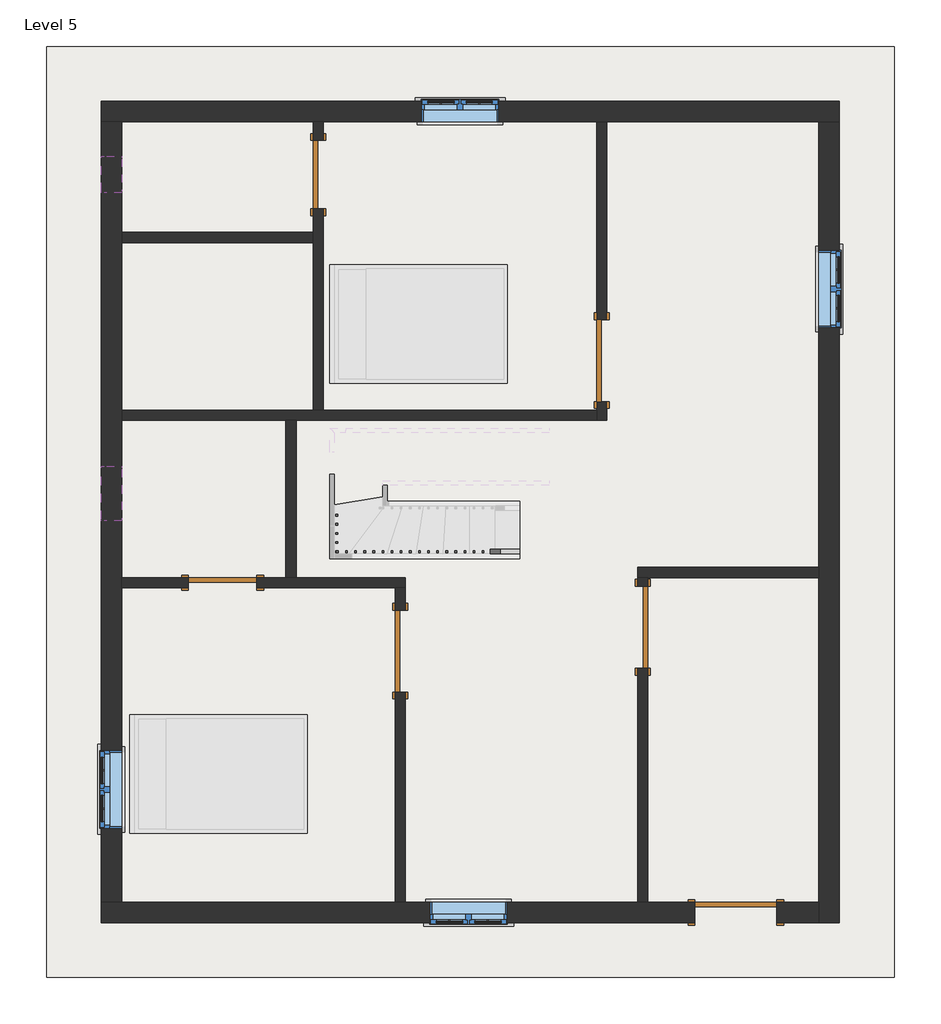
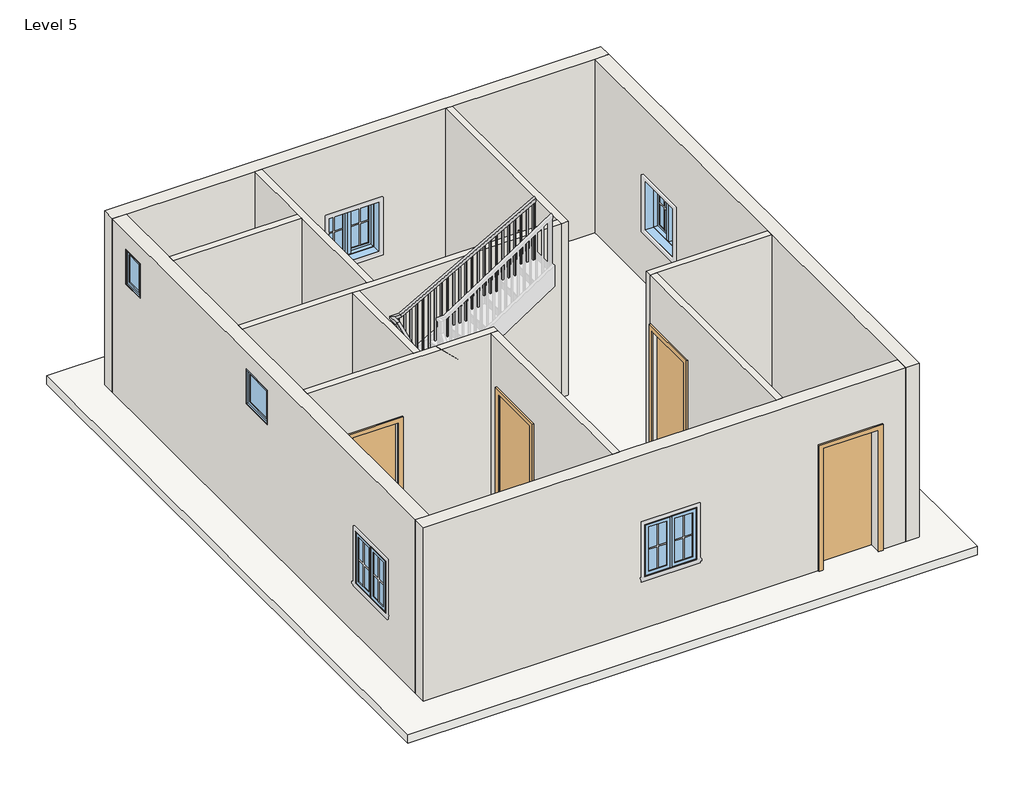
# One storey, part 1 of 2: 13 walls, 6 doors, 6 windows, 1 railing, 1 roof.
"""IFC4 building model written with IfcOpenShell, lengths in millimetres."""

from ifc_helpers import new_model, si_unit, frame, origin, place, context, project, spatial, polyline, outline, extrude, faceted_brep, transform, mapped, element, save
from components import door_d8f5dbb5, door_f2b275c1, door_305aa2a5, door_e5f9f3c4, door_0ca8825f, window_aa618e30, window_80340324, window_339605e1

model = new_model("IFC4")

# Units and contexts
model_context = context("Model", 3, world=origin())
ifc_project = project(units=[si_unit("LENGTHUNIT", "METRE", prefix="MILLI")], contexts=[model_context])

# Site, building, storey
site = spatial("IfcSite", under=ifc_project)
building = spatial("IfcBuilding", under=site)
storey = spatial("IfcBuildingStorey", under=building, Name="Level 5", Elevation=9601.2)

# Doors
placement = place(None, origin())
door_shape = door_d8f5dbb5(model_context)
element("IfcDoor", 1, ObjectType="Single-Flush : 30\" x 80\"", at=placement, inside=storey, context=model_context, shape_type="MappedRepresentation", body=[
    mapped(door_shape, transform((-2510.1648498, 3958.5558073, 9601.2), x_axis=(0.0, 1.0, 0.0), y_axis=(-1.0, 0.0, 0.0), z_axis=(0.0, 0.0, 1.0))),
])
door_2_shape = door_f2b275c1(model_context)
element("IfcDoor", 2, ObjectType="Single-Flush : 30\" x 80\"", at=placement, inside=storey, context=model_context, shape_type="MappedRepresentation", body=[
    mapped(door_2_shape, transform((-3576.9648498, -592.8066927, 9601.2), x_axis=(-1.0, 0.0, 0.0), y_axis=(0.0, -1.0, 0.0), z_axis=(0.0, 0.0, 1.0))),
])
door_3_shape = door_305aa2a5(model_context)
element("IfcDoor", 3, ObjectType="Single-Flush : 36\" x 84\"", at=placement, inside=storey, context=model_context, shape_type="MappedRepresentation", body=[
    mapped(door_3_shape, transform((652.1351502, 1883.6933073, 9601.2), x_axis=(0.0, -1.0, 0.0), y_axis=(1.0, 0.0, 0.0), z_axis=(0.0, 0.0, 1.0))),
])
element("IfcDoor", 4, ObjectType="Single-Flush : 36\" x 84\"", at=placement, inside=storey, context=model_context, shape_type="MappedRepresentation", body=[
    mapped(door_3_shape, transform((1109.3351502, -1088.1066927, 9601.2), x_axis=(0.0, 1.0, 0.0), y_axis=(-1.0, 0.0, 0.0), z_axis=(0.0, 0.0, 1.0))),
])
door_4_shape = door_e5f9f3c4(model_context)
element("IfcDoor", 5, ObjectType="Single-Flush : 36\" x 84\"", at=placement, inside=storey, context=model_context, shape_type="MappedRepresentation", body=[
    mapped(door_4_shape, transform((-1595.7648498, -1354.8066927, 9601.2), x_axis=(0.0, 1.0, 0.0), y_axis=(-1.0, 0.0, 0.0), z_axis=(0.0, 0.0, 1.0))),
])
door_5_shape = door_0ca8825f(model_context)
element("IfcDoor", 6, ObjectType="Single-Flush : 36\" x 84\"", at=placement, inside=storey, context=model_context, shape_type="MappedRepresentation", body=[
    mapped(door_5_shape, transform((2147.5601502, -4269.4566927, 9601.2), x_axis=(1.0, 0.0, 0.0), y_axis=(0.0, 1.0, 0.0), z_axis=(0.0, 0.0, 1.0))),
])

# Railing
element("IfcRailing", 7, ObjectType="Handrail - Rectangular", at=placement, inside=storey, context=model_context, shape_type="SolidModel", body=[
    faceted_brep([(-264.8831579, -271.8029286, 10684.9333333), (-264.8831579, -271.8029286, 10627.3518622), (-264.8831579, -221.0029286, 10627.3518622), (-264.8831579, -221.0029286, 10684.9333333), (-2203.3957557, -271.8029286, 11719.466441), (-2216.1029055, -271.8029286, 11668.666441), (-2216.1029055, -221.0029286, 11668.666441), (-2203.3957557, -221.0029286, 11719.466441), (-2328.8610857, -271.8029286, 11719.466441), (-2328.8610857, -271.8029286, 11668.666441), (-2278.0610857, -221.0029286, 11668.666441), (-2278.0610857, -221.0029286, 11719.466441), (-2328.8610857, -117.3180853, 11719.466441), (-2328.8610857, -107.2249429, 11668.666441), (-2278.0610857, -107.2249429, 11668.666441), (-2278.0610857, -117.3180853, 11719.466441), (-2328.8610857, 889.2076495, 12135.8648193), (-2328.8610857, 899.300792, 12085.0648193), (-2278.0610857, 899.300792, 12085.0648193), (-2278.0610857, 889.2076495, 12135.8648193), (-2328.8610857, 1080.0895433, 12135.8648193), (-2328.8610857, 1080.0895433, 12085.0648193), (-2278.0610857, 1029.2895433, 12085.0648193), (-2278.0610857, 1029.2895433, 12135.8648193), (-2181.3423106, 1080.0895433, 12135.8648193), (-2168.0744201, 1080.0895433, 12085.0648193), (-2168.0744201, 1029.2895433, 12085.0648193), (-2181.3423106, 1029.2895433, 12135.8648193), (63.4034409, 1080.0895433, 13394.2666667), (63.4034409, 1029.2895433, 13394.2666667), (63.4034409, 1029.2895433, 13336.0287027), (63.4034409, 1080.0895433, 13336.0287027)], [[[0, 1, 2, 3]], [[1, 0, 4, 5]], [[2, 1, 5, 6]], [[3, 2, 6, 7]], [[0, 3, 7, 4]], [[5, 4, 8, 9]], [[6, 5, 9, 10]], [[7, 6, 10, 11]], [[4, 7, 11, 8]], [[9, 8, 12, 13]], [[10, 9, 13, 14]], [[11, 10, 14, 15]], [[8, 11, 15, 12]], [[13, 12, 16, 17]], [[14, 13, 17, 18]], [[15, 14, 18, 19]], [[12, 15, 19, 16]], [[17, 16, 20, 21]], [[18, 17, 21, 22]], [[19, 18, 22, 23]], [[16, 19, 23, 20]], [[21, 20, 24, 25]], [[22, 21, 25, 26]], [[23, 22, 26, 27]], [[20, 23, 27, 24]], [[28, 29, 30, 31]], [[25, 24, 28, 31]], [[26, 25, 31, 30]], [[27, 26, 30, 29]], [[24, 27, 29, 28]]]),
    extrude(outline(polyline([(13313.8348603, 23.8139143), (12310.5333333, 23.8139143), (12310.5333333, 42.8639143), (13324.5142681, 42.8639143), (13313.8348603, 23.8139143)])), frame((0.0, 1045.1645433, 0.0), z_axis=(0.0, 1.0, 0.0), x_axis=(0.0, 0.0, 1.0)), (0.0, 0.0, 1.0), 19.05),
    extrude(outline(polyline([(13256.878019, -77.7860857), (12310.5333333, -77.7860857), (12310.5333333, -58.7360857), (13267.5574267, -58.7360857), (13256.878019, -77.7860857)])), frame((0.0, 1045.1645433, 0.0), z_axis=(0.0, 1.0, 0.0), x_axis=(0.0, 0.0, 1.0)), (0.0, 0.0, 1.0), 19.05),
    extrude(outline(polyline([(13199.9211776, -179.3860857), (12310.5333333, -179.3860857), (12310.5333333, -160.3360857), (13210.6005853, -160.3360857), (13199.9211776, -179.3860857)])), frame((0.0, 1045.1645433, 0.0), z_axis=(0.0, 1.0, 0.0), x_axis=(0.0, 0.0, 1.0)), (0.0, 0.0, 1.0), 19.05),
    extrude(outline(polyline([(13142.9643362, -280.9860857), (12141.2, -280.9860857), (12141.2, -261.9360857), (13153.643744, -261.9360857), (13142.9643362, -280.9860857)])), frame((0.0, 1045.1645433, 0.0), z_axis=(0.0, 1.0, 0.0), x_axis=(0.0, 0.0, 1.0)), (0.0, 0.0, 1.0), 19.05),
    extrude(outline(polyline([(13086.0074948, -382.5860857), (12141.2, -382.5860857), (12141.2, -363.5360857), (13096.6869026, -363.5360857), (13086.0074948, -382.5860857)])), frame((0.0, 1045.1645433, 0.0), z_axis=(0.0, 1.0, 0.0), x_axis=(0.0, 0.0, 1.0)), (0.0, 0.0, 1.0), 19.05),
    extrude(outline(polyline([(13029.0506535, -484.1860857), (12141.2, -484.1860857), (12141.2, -465.1360857), (13039.7300612, -465.1360857), (13029.0506535, -484.1860857)])), frame((0.0, 1045.1645433, 0.0), z_axis=(0.0, 1.0, 0.0), x_axis=(0.0, 0.0, 1.0)), (0.0, 0.0, 1.0), 19.05),
    extrude(outline(polyline([(12972.0938121, -585.7860857), (11971.8666667, -585.7860857), (11971.8666667, -566.7360857), (12982.7732198, -566.7360857), (12972.0938121, -585.7860857)])), frame((0.0, 1045.1645433, 0.0), z_axis=(0.0, 1.0, 0.0), x_axis=(0.0, 0.0, 1.0)), (0.0, 0.0, 1.0), 19.05),
    extrude(outline(polyline([(12915.1369707, -687.3860857), (11971.8666667, -687.3860857), (11971.8666667, -668.3360857), (12925.8163785, -668.3360857), (12915.1369707, -687.3860857)])), frame((0.0, 1045.1645433, 0.0), z_axis=(0.0, 1.0, 0.0), x_axis=(0.0, 0.0, 1.0)), (0.0, 0.0, 1.0), 19.05),
    extrude(outline(polyline([(12858.1801293, -788.9860857), (11971.8666667, -788.9860857), (11971.8666667, -769.9360857), (12868.8595371, -769.9360857), (12858.1801293, -788.9860857)])), frame((0.0, 1045.1645433, 0.0), z_axis=(0.0, 1.0, 0.0), x_axis=(0.0, 0.0, 1.0)), (0.0, 0.0, 1.0), 19.05),
    extrude(outline(polyline([(12801.223288, -890.5860857), (11802.5333333, -890.5860857), (11802.5333333, -871.5360857), (12811.9026957, -871.5360857), (12801.223288, -890.5860857)])), frame((0.0, 1045.1645433, 0.0), z_axis=(0.0, 1.0, 0.0), x_axis=(0.0, 0.0, 1.0)), (0.0, 0.0, 1.0), 19.05),
    extrude(outline(polyline([(12744.2664466, -992.1860857), (11802.5333333, -992.1860857), (11802.5333333, -973.1360857), (12754.9458543, -973.1360857), (12744.2664466, -992.1860857)])), frame((0.0, 1045.1645433, 0.0), z_axis=(0.0, 1.0, 0.0), x_axis=(0.0, 0.0, 1.0)), (0.0, 0.0, 1.0), 19.05),
    extrude(outline(polyline([(12687.3096052, -1093.7860857), (11633.2, -1093.7860857), (11633.2, -1074.7360857), (12697.989013, -1074.7360857), (12687.3096052, -1093.7860857)])), frame((0.0, 1045.1645433, 0.0), z_axis=(0.0, 1.0, 0.0), x_axis=(0.0, 0.0, 1.0)), (0.0, 0.0, 1.0), 19.05),
    extrude(outline(polyline([(12630.3527638, -1195.3860857), (11633.2, -1195.3860857), (11633.2, -1176.3360857), (12641.0321716, -1176.3360857), (12630.3527638, -1195.3860857)])), frame((0.0, 1045.1645433, 0.0), z_axis=(0.0, 1.0, 0.0), x_axis=(0.0, 0.0, 1.0)), (0.0, 0.0, 1.0), 19.05),
    extrude(outline(polyline([(12573.3959225, -1296.9860857), (11633.2, -1296.9860857), (11633.2, -1277.9360857), (12584.0753302, -1277.9360857), (12573.3959225, -1296.9860857)])), frame((0.0, 1045.1645433, 0.0), z_axis=(0.0, 1.0, 0.0), x_axis=(0.0, 0.0, 1.0)), (0.0, 0.0, 1.0), 19.05),
    extrude(outline(polyline([(12516.4390811, -1398.5860857), (11463.8666667, -1398.5860857), (11463.8666667, -1379.5360857), (12527.1184889, -1379.5360857), (12516.4390811, -1398.5860857)])), frame((0.0, 1045.1645433, 0.0), z_axis=(0.0, 1.0, 0.0), x_axis=(0.0, 0.0, 1.0)), (0.0, 0.0, 1.0), 19.05),
    extrude(outline(polyline([(12459.4822397, -1500.1860857), (11463.8666667, -1500.1860857), (11463.8666667, -1481.1360857), (12470.1616475, -1481.1360857), (12459.4822397, -1500.1860857)])), frame((0.0, 1045.1645433, 0.0), z_axis=(0.0, 1.0, 0.0), x_axis=(0.0, 0.0, 1.0)), (0.0, 0.0, 1.0), 19.05),
    extrude(outline(polyline([(12402.5253983, -1601.7860857), (11463.8666667, -1601.7860857), (11463.8666667, -1582.7360857), (12413.2048061, -1582.7360857), (12402.5253983, -1601.7860857)])), frame((0.0, 1045.1645433, 0.0), z_axis=(0.0, 1.0, 0.0), x_axis=(0.0, 0.0, 1.0)), (0.0, 0.0, 1.0), 19.05),
    extrude(outline(polyline([(12345.568557, -1703.3860857), (11294.5333333, -1703.3860857), (11294.5333333, -1684.3360857), (12356.2479647, -1684.3360857), (12345.568557, -1703.3860857)])), frame((0.0, 1045.1645433, 0.0), z_axis=(0.0, 1.0, 0.0), x_axis=(0.0, 0.0, 1.0)), (0.0, 0.0, 1.0), 19.05),
    extrude(outline(polyline([(12288.6117156, -1804.9860857), (11294.5333333, -1804.9860857), (11294.5333333, -1785.9360857), (12299.2911234, -1785.9360857), (12288.6117156, -1804.9860857)])), frame((0.0, 1045.1645433, 0.0), z_axis=(0.0, 1.0, 0.0), x_axis=(0.0, 0.0, 1.0)), (0.0, 0.0, 1.0), 19.05),
    extrude(outline(polyline([(12231.6548742, -1906.5860857), (11294.5333333, -1906.5860857), (11294.5333333, -1887.5360857), (12242.334282, -1887.5360857), (12231.6548742, -1906.5860857)])), frame((0.0, 1045.1645433, 0.0), z_axis=(0.0, 1.0, 0.0), x_axis=(0.0, 0.0, 1.0)), (0.0, 0.0, 1.0), 19.05),
    extrude(outline(polyline([(12174.6980329, -2008.1860857), (11294.5333333, -2008.1860857), (11294.5333333, -1989.1360857), (12185.3774406, -1989.1360857), (12174.6980329, -2008.1860857)])), frame((0.0, 1045.1645433, 0.0), z_axis=(0.0, 1.0, 0.0), x_axis=(0.0, 0.0, 1.0)), (0.0, 0.0, 1.0), 19.05),
    extrude(outline(polyline([(12117.7411915, -2109.7860857), (11125.2, -2109.7860857), (11125.2, -2090.7360857), (12128.4205992, -2090.7360857), (12117.7411915, -2109.7860857)])), frame((0.0, 1045.1645433, 0.0), z_axis=(0.0, 1.0, 0.0), x_axis=(0.0, 0.0, 1.0)), (0.0, 0.0, 1.0), 19.05),
    extrude(outline(polyline([(-2211.3860857, 1064.2145433), (-2192.3360857, 1064.2145433), (-2192.3360857, 1045.1645433), (-2211.3860857, 1045.1645433), (-2211.3860857, 1064.2145433)])), frame((0.0, 0.0, 11125.2), z_axis=(0.0, 0.0, 1.0), x_axis=(1.0, 0.0, 0.0)), (0.0, 0.0, 1.0), 959.8648193),
    extrude(outline(polyline([(-2312.9860857, 963.2720714), (-2312.9860857, 982.3220714), (-2293.9360857, 982.3220714), (-2293.9360857, 963.2720714), (-2312.9860857, 963.2720714)])), frame((0.0, 0.0, 11125.2), z_axis=(0.0, 0.0, 1.0), x_axis=(1.0, 0.0, 0.0)), (0.0, 0.0, 1.0), 959.8648193),
    extrude(outline(polyline([(880.7220714, 12077.3788269), (880.7220714, 11125.2), (861.6720714, 11125.2), (861.6720714, 12069.4978669), (880.7220714, 12077.3788269)])), frame((-2312.9860857, 0.0, 0.0), z_axis=(1.0, 0.0, 0.0), x_axis=(0.0, 1.0, 0.0)), (0.0, 0.0, 1.0), 19.05),
    extrude(outline(polyline([(779.1220714, 12035.34704), (779.1220714, 11125.2), (760.0720714, 11125.2), (760.0720714, 12027.4660799), (779.1220714, 12035.34704)])), frame((-2312.9860857, 0.0, 0.0), z_axis=(1.0, 0.0, 0.0), x_axis=(0.0, 1.0, 0.0)), (0.0, 0.0, 1.0), 19.05),
    extrude(outline(polyline([(677.5220714, 11993.315253), (677.5220714, 11125.2), (658.4720714, 11125.2), (658.4720714, 11985.434293), (677.5220714, 11993.315253)])), frame((-2312.9860857, 0.0, 0.0), z_axis=(1.0, 0.0, 0.0), x_axis=(0.0, 1.0, 0.0)), (0.0, 0.0, 1.0), 19.05),
    extrude(outline(polyline([(575.9220714, 11951.2834661), (575.9220714, 10955.8666667), (556.8720714, 10955.8666667), (556.8720714, 11943.402506), (575.9220714, 11951.2834661)])), frame((-2312.9860857, 0.0, 0.0), z_axis=(1.0, 0.0, 0.0), x_axis=(0.0, 1.0, 0.0)), (0.0, 0.0, 1.0), 19.05),
    extrude(outline(polyline([(474.3220714, 11909.2516792), (474.3220714, 10955.8666667), (455.2720714, 10955.8666667), (455.2720714, 11901.3707191), (474.3220714, 11909.2516792)])), frame((-2312.9860857, 0.0, 0.0), z_axis=(1.0, 0.0, 0.0), x_axis=(0.0, 1.0, 0.0)), (0.0, 0.0, 1.0), 19.05),
    extrude(outline(polyline([(372.7220714, 11867.2198922), (372.7220714, 10955.8666667), (353.6720714, 10955.8666667), (353.6720714, 11859.3389322), (372.7220714, 11867.2198922)])), frame((-2312.9860857, 0.0, 0.0), z_axis=(1.0, 0.0, 0.0), x_axis=(0.0, 1.0, 0.0)), (0.0, 0.0, 1.0), 19.05),
    extrude(outline(polyline([(271.1220714, 11825.1881053), (271.1220714, 10955.8666667), (252.0720714, 10955.8666667), (252.0720714, 11817.3071452), (271.1220714, 11825.1881053)])), frame((-2312.9860857, 0.0, 0.0), z_axis=(1.0, 0.0, 0.0), x_axis=(0.0, 1.0, 0.0)), (0.0, 0.0, 1.0), 19.05),
    extrude(outline(polyline([(169.5220714, 11783.1563183), (169.5220714, 10786.5333333), (150.4720714, 10786.5333333), (150.4720714, 11775.2753583), (169.5220714, 11783.1563183)])), frame((-2312.9860857, 0.0, 0.0), z_axis=(1.0, 0.0, 0.0), x_axis=(0.0, 1.0, 0.0)), (0.0, 0.0, 1.0), 19.05),
    extrude(outline(polyline([(67.9220714, 11741.1245314), (67.9220714, 10786.5333333), (48.8720714, 10786.5333333), (48.8720714, 11733.2435714), (67.9220714, 11741.1245314)])), frame((-2312.9860857, 0.0, 0.0), z_axis=(1.0, 0.0, 0.0), x_axis=(0.0, 1.0, 0.0)), (0.0, 0.0, 1.0), 19.05),
    extrude(outline(polyline([(-33.6779286, 11699.0927445), (-33.6779286, 10786.5333333), (-52.7279286, 10786.5333333), (-52.7279286, 11691.2117844), (-33.6779286, 11699.0927445)])), frame((-2312.9860857, 0.0, 0.0), z_axis=(1.0, 0.0, 0.0), x_axis=(0.0, 1.0, 0.0)), (0.0, 0.0, 1.0), 19.05),
    extrude(outline(polyline([(-2312.9860857, -154.3279286), (-2312.9860857, -135.2779286), (-2293.9360857, -135.2779286), (-2293.9360857, -154.3279286), (-2312.9860857, -154.3279286)])), frame((0.0, 0.0, 10786.5333333), z_axis=(0.0, 0.0, 1.0), x_axis=(1.0, 0.0, 0.0)), (0.0, 0.0, 1.0), 882.1331077),
    extrude(outline(polyline([(-2287.3581579, -255.9279286), (-2306.4081579, -255.9279286), (-2306.4081579, -236.8779286), (-2287.3581579, -236.8779286), (-2287.3581579, -255.9279286)])), frame((0.0, 0.0, 10786.5333333), z_axis=(0.0, 0.0, 1.0), x_axis=(1.0, 0.0, 0.0)), (0.0, 0.0, 1.0), 882.1331077),
    extrude(outline(polyline([(11662.6387317, -2204.8081579), (10786.5333333, -2204.8081579), (10786.5333333, -2185.7581579), (11652.4722486, -2185.7581579), (11662.6387317, -2204.8081579)])), frame((0.0, -255.9279286, 0.0), z_axis=(0.0, 1.0, 0.0), x_axis=(0.0, 0.0, 1.0)), (0.0, 0.0, 1.0), 19.05),
    extrude(outline(polyline([(11608.4174882, -2103.2081579), (10617.2, -2103.2081579), (10617.2, -2084.1581579), (11598.251005, -2084.1581579), (11608.4174882, -2103.2081579)])), frame((0.0, -255.9279286, 0.0), z_axis=(0.0, 1.0, 0.0), x_axis=(0.0, 0.0, 1.0)), (0.0, 0.0, 1.0), 19.05),
    extrude(outline(polyline([(11554.1962446, -2001.6081579), (10617.2, -2001.6081579), (10617.2, -1982.5581579), (11544.0297614, -1982.5581579), (11554.1962446, -2001.6081579)])), frame((0.0, -255.9279286, 0.0), z_axis=(0.0, 1.0, 0.0), x_axis=(0.0, 0.0, 1.0)), (0.0, 0.0, 1.0), 19.05),
    extrude(outline(polyline([(11499.975001, -1900.0081579), (10617.2, -1900.0081579), (10617.2, -1880.9581579), (11489.8085178, -1880.9581579), (11499.975001, -1900.0081579)])), frame((0.0, -255.9279286, 0.0), z_axis=(0.0, 1.0, 0.0), x_axis=(0.0, 0.0, 1.0)), (0.0, 0.0, 1.0), 19.05),
    extrude(outline(polyline([(11445.7537574, -1798.4081579), (10617.2, -1798.4081579), (10617.2, -1779.3581579), (11435.5872743, -1779.3581579), (11445.7537574, -1798.4081579)])), frame((0.0, -255.9279286, 0.0), z_axis=(0.0, 1.0, 0.0), x_axis=(0.0, 0.0, 1.0)), (0.0, 0.0, 1.0), 19.05),
    extrude(outline(polyline([(11391.5325139, -1696.8081579), (10447.8666667, -1696.8081579), (10447.8666667, -1677.7581579), (11381.3660307, -1677.7581579), (11391.5325139, -1696.8081579)])), frame((0.0, -255.9279286, 0.0), z_axis=(0.0, 1.0, 0.0), x_axis=(0.0, 0.0, 1.0)), (0.0, 0.0, 1.0), 19.05),
    extrude(outline(polyline([(11337.3112703, -1595.2081579), (10447.8666667, -1595.2081579), (10447.8666667, -1576.1581579), (11327.1447871, -1576.1581579), (11337.3112703, -1595.2081579)])), frame((0.0, -255.9279286, 0.0), z_axis=(0.0, 1.0, 0.0), x_axis=(0.0, 0.0, 1.0)), (0.0, 0.0, 1.0), 19.05),
    extrude(outline(polyline([(11283.0900267, -1493.6081579), (10447.8666667, -1493.6081579), (10447.8666667, -1474.5581579), (11272.9235435, -1474.5581579), (11283.0900267, -1493.6081579)])), frame((0.0, -255.9279286, 0.0), z_axis=(0.0, 1.0, 0.0), x_axis=(0.0, 0.0, 1.0)), (0.0, 0.0, 1.0), 19.05),
    extrude(outline(polyline([(11228.8687831, -1392.0081579), (10278.5333333, -1392.0081579), (10278.5333333, -1372.9581579), (11218.7023, -1372.9581579), (11228.8687831, -1392.0081579)])), frame((0.0, -255.9279286, 0.0), z_axis=(0.0, 1.0, 0.0), x_axis=(0.0, 0.0, 1.0)), (0.0, 0.0, 1.0), 19.05),
    extrude(outline(polyline([(11174.6475396, -1290.4081579), (10278.5333333, -1290.4081579), (10278.5333333, -1271.3581579), (11164.4810564, -1271.3581579), (11174.6475396, -1290.4081579)])), frame((0.0, -255.9279286, 0.0), z_axis=(0.0, 1.0, 0.0), x_axis=(0.0, 0.0, 1.0)), (0.0, 0.0, 1.0), 19.05),
    extrude(outline(polyline([(11120.426296, -1188.8081579), (10278.5333333, -1188.8081579), (10278.5333333, -1169.7581579), (11110.2598128, -1169.7581579), (11120.426296, -1188.8081579)])), frame((0.0, -255.9279286, 0.0), z_axis=(0.0, 1.0, 0.0), x_axis=(0.0, 0.0, 1.0)), (0.0, 0.0, 1.0), 19.05),
    extrude(outline(polyline([(11066.2050524, -1087.2081579), (10109.2, -1087.2081579), (10109.2, -1068.1581579), (11056.0385692, -1068.1581579), (11066.2050524, -1087.2081579)])), frame((0.0, -255.9279286, 0.0), z_axis=(0.0, 1.0, 0.0), x_axis=(0.0, 0.0, 1.0)), (0.0, 0.0, 1.0), 19.05),
    extrude(outline(polyline([(11011.9838088, -985.6081579), (10109.2, -985.6081579), (10109.2, -966.5581579), (11001.8173257, -966.5581579), (11011.9838088, -985.6081579)])), frame((0.0, -255.9279286, 0.0), z_axis=(0.0, 1.0, 0.0), x_axis=(0.0, 0.0, 1.0)), (0.0, 0.0, 1.0), 19.05),
    extrude(outline(polyline([(10957.7625653, -884.0081579), (10109.2, -884.0081579), (10109.2, -864.9581579), (10947.5960821, -864.9581579), (10957.7625653, -884.0081579)])), frame((0.0, -255.9279286, 0.0), z_axis=(0.0, 1.0, 0.0), x_axis=(0.0, 0.0, 1.0)), (0.0, 0.0, 1.0), 19.05),
    extrude(outline(polyline([(10903.5413217, -782.4081579), (9939.8666667, -782.4081579), (9939.8666667, -763.3581579), (10893.3748385, -763.3581579), (10903.5413217, -782.4081579)])), frame((0.0, -255.9279286, 0.0), z_axis=(0.0, 1.0, 0.0), x_axis=(0.0, 0.0, 1.0)), (0.0, 0.0, 1.0), 19.05),
    extrude(outline(polyline([(10849.3200781, -680.8081579), (9939.8666667, -680.8081579), (9939.8666667, -661.7581579), (10839.1535949, -661.7581579), (10849.3200781, -680.8081579)])), frame((0.0, -255.9279286, 0.0), z_axis=(0.0, 1.0, 0.0), x_axis=(0.0, 0.0, 1.0)), (0.0, 0.0, 1.0), 19.05),
    extrude(outline(polyline([(10795.0988345, -579.2081579), (9939.8666667, -579.2081579), (9939.8666667, -560.1581579), (10784.9323514, -560.1581579), (10795.0988345, -579.2081579)])), frame((0.0, -255.9279286, 0.0), z_axis=(0.0, 1.0, 0.0), x_axis=(0.0, 0.0, 1.0)), (0.0, 0.0, 1.0), 19.05),
    extrude(outline(polyline([(10740.877591, -477.6081579), (9770.5333333, -477.6081579), (9770.5333333, -458.5581579), (10730.7111078, -458.5581579), (10740.877591, -477.6081579)])), frame((0.0, -255.9279286, 0.0), z_axis=(0.0, 1.0, 0.0), x_axis=(0.0, 0.0, 1.0)), (0.0, 0.0, 1.0), 19.05),
    extrude(outline(polyline([(10686.6563474, -376.0081579), (9770.5333333, -376.0081579), (9770.5333333, -356.9581579), (10676.4898642, -356.9581579), (10686.6563474, -376.0081579)])), frame((0.0, -255.9279286, 0.0), z_axis=(0.0, 1.0, 0.0), x_axis=(0.0, 0.0, 1.0)), (0.0, 0.0, 1.0), 19.05),
    extrude(outline(polyline([(-2312.9860857, 1045.1645433), (-2312.9860857, 1064.2145433), (-2293.9360857, 1064.2145433), (-2293.9360857, 1045.1645433), (-2312.9860857, 1045.1645433)])), frame((0.0, 0.0, 11125.2), z_axis=(0.0, 0.0, 1.0), x_axis=(1.0, 0.0, 0.0)), (0.0, 0.0, 1.0), 959.8648193),
    extrude(outline(polyline([(-2293.9360857, -255.9279286), (-2312.9860857, -255.9279286), (-2312.9860857, -236.8779286), (-2293.9360857, -236.8779286), (-2293.9360857, -255.9279286)])), frame((0.0, 0.0, 10786.5333333), z_axis=(0.0, 0.0, 1.0), x_axis=(1.0, 0.0, 0.0)), (0.0, 0.0, 1.0), 882.1331077),
    extrude(outline(polyline([(13325.349295, 44.3534409), (12310.5333333, 44.3534409), (12310.5333333, 63.4034409), (13336.0287027, 63.4034409), (13325.349295, 44.3534409)])), frame((0.0, 1045.1645433, 0.0), z_axis=(0.0, 1.0, 0.0), x_axis=(0.0, 0.0, 1.0)), (0.0, 0.0, 1.0), 19.05),
    extrude(outline(polyline([(10637.5183454, -283.9331579), (9770.5333333, -283.9331579), (9770.5333333, -264.8831579), (10627.3518622, -264.8831579), (10637.5183454, -283.9331579)])), frame((0.0, -255.9279286, 0.0), z_axis=(0.0, 1.0, 0.0), x_axis=(0.0, 0.0, 1.0)), (0.0, 0.0, 1.0), 19.05),
])

# Roof
element("IfcRoof", 8, ObjectType="Generic - 12\"", at=placement, inside=storey, context=model_context, shape_type="SweptSolid", body=[
    extrude(outline(polyline([(-5539.1148498, 5385.7183073), (3909.6851502, 5385.7183073), (3909.6851502, -4993.3566927), (-5539.1148498, -4993.3566927), (-5539.1148498, 5385.7183073)])), frame((0.0, 0.0, 9448.8), z_axis=(0.0, 0.0, 1.0), x_axis=(1.0, 0.0, 0.0)), (0.0, 0.0, 1.0), 152.4),
])

# Walls
element("IfcWall", 9, ObjectType="WALL4.5\"", at=placement, inside=storey, context=model_context, shape_type="SweptSolid", body=[
    extrude(outline(polyline([(-2567.3148498, 3198.1433073), (-4700.9148498, 3198.1433073), (-4700.9148498, 3312.4433073), (-2567.3148498, 3312.4433073), (-2567.3148498, 3198.1433073)])), frame((0.0, 0.0, 9601.2), z_axis=(0.0, 0.0, 1.0), x_axis=(1.0, 0.0, 0.0)), (0.0, 0.0, 1.0), 3048.0),
])
element("IfcWall", 10, ObjectType="WALL4.5\"", at=placement, inside=storey, context=model_context, shape_type="Brep", body=[
    faceted_brep([(-2567.3148498, 4547.5183073, 9601.2), (-2567.3148498, 4339.5558073, 9601.2), (-2567.3148498, 4339.5558073, 11633.2), (-2567.3148498, 3577.5558073, 11633.2), (-2567.3148498, 3577.5558073, 9601.2), (-2567.3148498, 3312.4433073, 9601.2), (-2567.3148498, 3198.1433073, 9601.2), (-2567.3148498, 1331.2433073, 9601.2), (-2567.3148498, 1331.2433073, 12649.2), (-2567.3148498, 3198.1433073, 12649.2), (-2567.3148498, 3312.4433073, 12649.2), (-2567.3148498, 4547.5183073, 12649.2), (-2453.0148498, 4339.5558073, 11633.2), (-2453.0148498, 4339.5558073, 9601.2), (-2453.0148498, 4547.5183073, 9601.2), (-2453.0148498, 4547.5183073, 12649.2), (-2453.0148498, 1331.2433073, 12649.2), (-2453.0148498, 1331.2433073, 9601.2), (-2453.0148498, 3577.5558073, 9601.2), (-2453.0148498, 3577.5558073, 11633.2)], [[[0, 1, 2, 3, 4, 5, 6, 7, 8, 9, 10, 11]], [[12, 13, 14, 15, 16, 17, 18, 19]], [[18, 17, 7, 6, 5, 4]], [[14, 13, 1, 0]], [[0, 11, 15, 14]], [[8, 7, 17, 16]], [[2, 1, 13, 12]], [[3, 2, 12, 19]], [[4, 3, 19, 18]], [[11, 10, 9, 8, 16, 15]]]),
])
element("IfcWall", 11, ObjectType="WALL4.5\"", at=placement, inside=storey, context=model_context, shape_type="Brep", body=[
    faceted_brep([(594.9851502, 1426.4933073, 11734.8), (594.9851502, 1426.4933073, 9601.2), (594.9851502, 1331.2433073, 9601.2), (594.9851502, 1216.9433073, 9601.2), (594.9851502, 1216.9433073, 12649.2), (594.9851502, 1331.2433073, 12649.2), (594.9851502, 4547.5183073, 12649.2), (594.9851502, 4547.5183073, 9601.2), (594.9851502, 2340.8933073, 9601.2), (594.9851502, 2340.8933073, 11734.8), (709.2851502, 1216.9433073, 9601.2), (709.2851502, 1426.4933073, 9601.2), (709.2851502, 1426.4933073, 11734.8), (709.2851502, 2340.8933073, 11734.8), (709.2851502, 2340.8933073, 9601.2), (709.2851502, 4547.5183073, 9601.2), (709.2851502, 4547.5183073, 12649.2), (709.2851502, 1216.9433073, 12649.2)], [[[0, 1, 2, 3, 4, 5, 6, 7, 8, 9]], [[10, 11, 12, 13, 14, 15, 16, 17]], [[8, 7, 15, 14]], [[3, 2, 1, 11, 10]], [[7, 6, 16, 15]], [[4, 3, 10, 17]], [[12, 11, 1, 0]], [[13, 12, 0, 9]], [[14, 13, 9, 8]], [[6, 5, 4, 17, 16]]]),
])
element("IfcWall", 12, ObjectType="WALL4.5\"", at=placement, inside=storey, context=model_context, shape_type="Brep", body=[
    faceted_brep([(-4700.9148498, 1216.9433073, 9601.2), (-2872.1148498, 1216.9433073, 9601.2), (-2757.8148498, 1216.9433073, 9601.2), (594.9851502, 1216.9433073, 9601.2), (594.9851502, 1216.9433073, 12649.2), (-2757.8148498, 1216.9433073, 12649.2), (-2872.1148498, 1216.9433073, 12649.2), (-4700.9148498, 1216.9433073, 12649.2), (-4700.9148498, 1331.2433073, 9601.2), (-4700.9148498, 1331.2433073, 12649.2), (-2567.3148498, 1331.2433073, 12649.2), (-2453.0148498, 1331.2433073, 12649.2), (594.9851502, 1331.2433073, 12649.2), (594.9851502, 1331.2433073, 9601.2), (-2453.0148498, 1331.2433073, 9601.2), (-2567.3148498, 1331.2433073, 9601.2)], [[[0, 1, 2, 3, 4, 5, 6, 7]], [[8, 9, 10, 11, 12, 13, 14, 15]], [[3, 2, 1, 0, 8, 15, 14, 13]], [[4, 3, 13, 12]], [[0, 7, 9, 8]], [[7, 6, 5, 4, 12, 11, 10, 9]]]),
])
element("IfcWall", 13, ObjectType="WALL4.5\"", at=placement, inside=storey, context=model_context, shape_type="SweptSolid", body=[
    extrude(outline(polyline([(-2872.1148498, -535.6566927), (-2872.1148498, 1216.9433073), (-2757.8148498, 1216.9433073), (-2757.8148498, -535.6566927), (-2872.1148498, -535.6566927)])), frame((0.0, 0.0, 9601.2), z_axis=(0.0, 0.0, 1.0), x_axis=(1.0, 0.0, 0.0)), (0.0, 0.0, 1.0), 3048.0),
])
element("IfcWall", 14, ObjectType="WALL4.5\"", at=placement, inside=storey, context=model_context, shape_type="Brep", body=[
    faceted_brep([(-4700.9148498, -649.9566927, 9601.2), (-3957.9648498, -649.9566927, 9601.2), (-3957.9648498, -649.9566927, 11633.2), (-3195.9648498, -649.9566927, 11633.2), (-3195.9648498, -649.9566927, 9601.2), (-1652.9148498, -649.9566927, 9601.2), (-1538.6148498, -649.9566927, 9601.2), (-1538.6148498, -649.9566927, 12649.2), (-1652.9148498, -649.9566927, 12649.2), (-4700.9148498, -649.9566927, 12649.2), (-3957.9648498, -535.6566927, 11633.2), (-3957.9648498, -535.6566927, 9601.2), (-4700.9148498, -535.6566927, 9601.2), (-4700.9148498, -535.6566927, 12649.2), (-2872.1148498, -535.6566927, 12649.2), (-2757.8148498, -535.6566927, 12649.2), (-1538.6148498, -535.6566927, 12649.2), (-1538.6148498, -535.6566927, 9601.2), (-2757.8148498, -535.6566927, 9601.2), (-2872.1148498, -535.6566927, 9601.2), (-3195.9648498, -535.6566927, 9601.2), (-3195.9648498, -535.6566927, 11633.2)], [[[0, 1, 2, 3, 4, 5, 6, 7, 8, 9]], [[10, 11, 12, 13, 14, 15, 16, 17, 18, 19, 20, 21]], [[12, 11, 1, 0]], [[20, 19, 18, 17, 6, 5, 4]], [[7, 6, 17, 16]], [[0, 9, 13, 12]], [[2, 1, 11, 10]], [[3, 2, 10, 21]], [[4, 3, 21, 20]], [[9, 8, 7, 16, 15, 14, 13]]]),
])
element("IfcWall", 15, ObjectType="WALL4.5\"", at=placement, inside=storey, context=model_context, shape_type="Brep", body=[
    faceted_brep([(3071.4851502, -421.3566927, 9601.2), (1052.1851502, -421.3566927, 9601.2), (1052.1851502, -421.3566927, 12649.2), (3071.4851502, -421.3566927, 12649.2), (3071.4851502, -535.6566927, 9601.2), (3071.4851502, -535.6566927, 12649.2), (1166.4851502, -535.6566927, 12649.2), (1052.1851502, -535.6566927, 12649.2), (1052.1851502, -535.6566927, 9601.2), (1166.4851502, -535.6566927, 9601.2)], [[[0, 1, 2, 3]], [[4, 5, 6, 7, 8, 9]], [[1, 0, 4, 9, 8]], [[0, 3, 5, 4]], [[2, 1, 8, 7]], [[3, 2, 7, 6, 5]]]),
])
element("IfcWall", 16, ObjectType="WALL4.5\"", at=placement, inside=storey, context=model_context, shape_type="SweptSolid", body=[
    extrude(outline(polyline([(-535.6566927, 9601.2), (-630.9066927, 9601.2), (-630.9066927, 11734.8), (-1545.3066927, 11734.8), (-1545.3066927, 9601.2), (-4155.1566927, 9601.2), (-4155.1566927, 12649.2), (-535.6566927, 12649.2), (-535.6566927, 9601.2)])), frame((1052.1851502, 0.0, 0.0), z_axis=(1.0, 0.0, 0.0), x_axis=(0.0, 1.0, 0.0)), (0.0, 0.0, 1.0), 114.3),
])
element("IfcWall", 17, ObjectType="WALL4.5\"", at=placement, inside=storey, context=model_context, shape_type="SweptSolid", body=[
    extrude(outline(polyline([(-649.9566927, 9601.2), (-897.6066927, 9601.2), (-897.6066927, 11734.8), (-1812.0066927, 11734.8), (-1812.0066927, 9601.2), (-4155.1566927, 9601.2), (-4155.1566927, 12649.2), (-649.9566927, 12649.2), (-649.9566927, 9601.2)])), frame((-1652.9148498, 0.0, 0.0), z_axis=(1.0, 0.0, 0.0), x_axis=(0.0, 1.0, 0.0)), (0.0, 0.0, 1.0), 114.3),
])
element("IfcWall", 18, ObjectType="WALL9\"", at=placement, inside=storey, context=model_context, shape_type="Brep", body=[
    faceted_brep([(-4929.5148498, 4547.5183073, 9601.2), (-4700.9148498, 4547.5183073, 9601.2), (-2567.3148498, 4547.5183073, 9601.2), (-2453.0148498, 4547.5183073, 9601.2), (594.9851502, 4547.5183073, 9601.2), (709.2851502, 4547.5183073, 9601.2), (3071.4851502, 4547.5183073, 9601.2), (3300.0851502, 4547.5183073, 9601.2), (3300.0851502, 4547.5183073, 12649.2), (3071.4851502, 4547.5183073, 12649.2), (709.2851502, 4547.5183073, 12649.2), (594.9851502, 4547.5183073, 12649.2), (-2453.0148498, 4547.5183073, 12649.2), (-2567.3148498, 4547.5183073, 12649.2), (-4700.9148498, 4547.5183073, 12649.2), (-4929.5148498, 4547.5183073, 12649.2), (-497.2148498, 4547.5183073, 11430.0), (-497.2148498, 4547.5183073, 10515.6), (-1360.8148498, 4547.5183073, 10515.6), (-1360.8148498, 4547.5183073, 11430.0), (-4929.5148498, 4776.1183073, 9601.2), (-4929.5148498, 4776.1183073, 12649.2), (3300.0851502, 4776.1183073, 12649.2), (3300.0851502, 4776.1183073, 9601.2), (-497.2148498, 4776.1183073, 11430.0), (-1360.8148498, 4776.1183073, 11430.0), (-1360.8148498, 4776.1183073, 10515.6), (-497.2148498, 4776.1183073, 10515.6)], [[[0, 1, 2, 3, 4, 5, 6, 7, 8, 9, 10, 11, 12, 13, 14, 15], [16, 17, 18, 19]], [[20, 21, 22, 23], [24, 25, 26, 27]], [[7, 6, 5, 4, 3, 2, 1, 0, 20, 23]], [[8, 7, 23, 22]], [[0, 15, 21, 20]], [[17, 16, 24, 27]], [[18, 17, 27, 26]], [[19, 18, 26, 25]], [[16, 19, 25, 24]], [[15, 14, 13, 12, 11, 10, 9, 8, 22, 21]]]),
])
element("IfcWall", 19, ObjectType="WALL9\"", at=placement, inside=storey, context=model_context, shape_type="Brep", body=[
    faceted_brep([(3071.4851502, 4547.5183073, 9601.2), (3071.4851502, -421.3566927, 9601.2), (3071.4851502, -535.6566927, 9601.2), (3071.4851502, -4155.1566927, 9601.2), (3071.4851502, -4383.7566927, 9601.2), (3071.4851502, -4383.7566927, 12649.2), (3071.4851502, -4155.1566927, 12649.2), (3071.4851502, -535.6566927, 12649.2), (3071.4851502, -421.3566927, 12649.2), (3071.4851502, 4547.5183073, 12649.2), (3071.4851502, 2248.8183073, 11430.0), (3071.4851502, 2248.8183073, 10515.6), (3071.4851502, 3112.4183073, 10515.6), (3071.4851502, 3112.4183073, 11430.0), (3300.0851502, 4547.5183073, 9601.2), (3300.0851502, 4547.5183073, 12649.2), (3300.0851502, -4383.7566927, 12649.2), (3300.0851502, -4383.7566927, 9601.2), (3300.0851502, 2248.8183073, 11430.0), (3300.0851502, 3112.4183073, 11430.0), (3300.0851502, 3112.4183073, 10515.6), (3300.0851502, 2248.8183073, 10515.6)], [[[0, 1, 2, 3, 4, 5, 6, 7, 8, 9], [10, 11, 12, 13]], [[14, 15, 16, 17], [18, 19, 20, 21]], [[4, 3, 2, 1, 0, 14, 17]], [[0, 9, 15, 14]], [[5, 4, 17, 16]], [[11, 10, 18, 21]], [[12, 11, 21, 20]], [[13, 12, 20, 19]], [[10, 13, 19, 18]], [[9, 8, 7, 6, 5, 16, 15]]]),
])
element("IfcWall", 20, ObjectType="WALL9\"", at=placement, inside=storey, context=model_context, shape_type="Brep", body=[
    faceted_brep([(3071.4851502, -4155.1566927, 9601.2), (2604.7601502, -4155.1566927, 9601.2), (2604.7601502, -4155.1566927, 11734.8), (1690.3601502, -4155.1566927, 11734.8), (1690.3601502, -4155.1566927, 9601.2), (1166.4851502, -4155.1566927, 9601.2), (1052.1851502, -4155.1566927, 9601.2), (-1538.6148498, -4155.1566927, 9601.2), (-1652.9148498, -4155.1566927, 9601.2), (-4700.9148498, -4155.1566927, 9601.2), (-4929.5148498, -4155.1566927, 9601.2), (-4929.5148498, -4155.1566927, 12649.2), (-4700.9148498, -4155.1566927, 12649.2), (-1652.9148498, -4155.1566927, 12649.2), (-1538.6148498, -4155.1566927, 12649.2), (1052.1851502, -4155.1566927, 12649.2), (1166.4851502, -4155.1566927, 12649.2), (3071.4851502, -4155.1566927, 12649.2), (-1265.5648498, -4155.1566927, 11430.0), (-1265.5648498, -4155.1566927, 10515.6), (-401.9648498, -4155.1566927, 10515.6), (-401.9648498, -4155.1566927, 11430.0), (2604.7601502, -4383.7566927, 11734.8), (2604.7601502, -4383.7566927, 9601.2), (3071.4851502, -4383.7566927, 9601.2), (3071.4851502, -4383.7566927, 12649.2), (-4929.5148498, -4383.7566927, 12649.2), (-4929.5148498, -4383.7566927, 9601.2), (1690.3601502, -4383.7566927, 9601.2), (1690.3601502, -4383.7566927, 11734.8), (-1265.5648498, -4383.7566927, 11430.0), (-401.9648498, -4383.7566927, 11430.0), (-401.9648498, -4383.7566927, 10515.6), (-1265.5648498, -4383.7566927, 10515.6)], [[[0, 1, 2, 3, 4, 5, 6, 7, 8, 9, 10, 11, 12, 13, 14, 15, 16, 17], [18, 19, 20, 21]], [[22, 23, 24, 25, 26, 27, 28, 29], [30, 31, 32, 33]], [[28, 27, 10, 9, 8, 7, 6, 5, 4]], [[24, 23, 1, 0]], [[0, 17, 25, 24]], [[11, 10, 27, 26]], [[19, 18, 30, 33]], [[20, 19, 33, 32]], [[21, 20, 32, 31]], [[18, 21, 31, 30]], [[17, 16, 15, 14, 13, 12, 11, 26, 25]], [[2, 1, 23, 22]], [[3, 2, 22, 29]], [[4, 3, 29, 28]]]),
])
element("IfcWall", 21, ObjectType="WALL9\"", at=placement, inside=storey, context=model_context, shape_type="Brep", body=[
    faceted_brep([(-4700.9148498, -4155.1566927, 9601.2), (-4700.9148498, -649.9566927, 9601.2), (-4700.9148498, -535.6566927, 9601.2), (-4700.9148498, 1216.9433073, 9601.2), (-4700.9148498, 1331.2433073, 9601.2), (-4700.9148498, 3198.1433073, 9601.2), (-4700.9148498, 3312.4433073, 9601.2), (-4700.9148498, 4547.5183073, 9601.2), (-4700.9148498, 4547.5183073, 12649.2), (-4700.9148498, 3312.4433073, 12649.2), (-4700.9148498, 3198.1433073, 12649.2), (-4700.9148498, 1331.2433073, 12649.2), (-4700.9148498, 1216.9433073, 12649.2), (-4700.9148498, -535.6566927, 12649.2), (-4700.9148498, -649.9566927, 12649.2), (-4700.9148498, -4155.1566927, 12649.2), (-4700.9148498, 4161.7558073, 12344.4), (-4700.9148498, 4161.7558073, 11734.8), (-4700.9148498, 3755.3558073, 11734.8), (-4700.9148498, 3755.3558073, 12344.4), (-4700.9148498, 705.7683073, 12344.4), (-4700.9148498, 705.7683073, 11734.8), (-4700.9148498, 96.1683073, 11734.8), (-4700.9148498, 96.1683073, 12344.4), (-4700.9148498, -2466.0566927, 11430.0), (-4700.9148498, -2466.0566927, 10515.6), (-4700.9148498, -3329.6566927, 10515.6), (-4700.9148498, -3329.6566927, 11430.0), (-4929.5148498, -4155.1566927, 9601.2), (-4929.5148498, -4155.1566927, 12649.2), (-4929.5148498, 4547.5183073, 12649.2), (-4929.5148498, 4547.5183073, 9601.2), (-4929.5148498, 4161.7558073, 12344.4), (-4929.5148498, 3755.3558073, 12344.4), (-4929.5148498, 3755.3558073, 11734.8), (-4929.5148498, 4161.7558073, 11734.8), (-4929.5148498, 705.7683073, 12344.4), (-4929.5148498, 96.1683073, 12344.4), (-4929.5148498, 96.1683073, 11734.8), (-4929.5148498, 705.7683073, 11734.8), (-4929.5148498, -2466.0566927, 11430.0), (-4929.5148498, -3329.6566927, 11430.0), (-4929.5148498, -3329.6566927, 10515.6), (-4929.5148498, -2466.0566927, 10515.6)], [[[0, 1, 2, 3, 4, 5, 6, 7, 8, 9, 10, 11, 12, 13, 14, 15], [16, 17, 18, 19], [20, 21, 22, 23], [24, 25, 26, 27]], [[28, 29, 30, 31], [32, 33, 34, 35], [36, 37, 38, 39], [40, 41, 42, 43]], [[7, 6, 5, 4, 3, 2, 1, 0, 28, 31]], [[8, 7, 31, 30]], [[0, 15, 29, 28]], [[17, 16, 32, 35]], [[18, 17, 35, 34]], [[19, 18, 34, 33]], [[16, 19, 33, 32]], [[21, 20, 36, 39]], [[22, 21, 39, 38]], [[23, 22, 38, 37]], [[20, 23, 37, 36]], [[25, 24, 40, 43]], [[26, 25, 43, 42]], [[27, 26, 42, 41]], [[24, 27, 41, 40]], [[15, 14, 13, 12, 11, 10, 9, 8, 30, 29]]]),
])

# Windows
window_shape = window_aa618e30(model_context)
element("IfcWindow", 22, ObjectType="Fixed : 16\" x 24\"", at=placement, inside=storey, context=model_context, shape_type="MappedRepresentation", body=[
    mapped(window_shape, transform((-4815.2148498, 3996.6558073, 10820.4), x_axis=(0.0, 1.0, 0.0), y_axis=(-1.0, 0.0, 0.0), z_axis=(0.0, 0.0, 1.0))),
])
window_2_shape = window_80340324(model_context)
element("IfcWindow", 23, ObjectType="Fixed : 24\" x 24\"", at=placement, inside=storey, context=model_context, shape_type="MappedRepresentation", body=[
    mapped(window_2_shape, transform((-4815.2148498, 439.0683073, 10820.4), x_axis=(0.0, 1.0, 0.0), y_axis=(-1.0, 0.0, 0.0), z_axis=(0.0, 0.0, 1.0))),
])
window_3_shape = window_339605e1(model_context)
element("IfcWindow", 24, ObjectType="Window-Casement-Double : 34\" x 36\"", at=placement, inside=storey, context=model_context, shape_type="MappedRepresentation", body=[
    mapped(window_3_shape, transform((-929.0148498, 4661.8183073, 9601.2), x_axis=(1.0, 0.0, 0.0), y_axis=(0.0, 1.0, 0.0), z_axis=(0.0, 0.0, 1.0))),
])
element("IfcWindow", 25, ObjectType="Window-Casement-Double : 34\" x 36\"", at=placement, inside=storey, context=model_context, shape_type="MappedRepresentation", body=[
    mapped(window_3_shape, transform((3185.7851502, 2680.6183073, 9601.2), x_axis=(0.0, -1.0, 0.0), y_axis=(1.0, 0.0, 0.0), z_axis=(0.0, 0.0, 1.0))),
])
element("IfcWindow", 26, ObjectType="Window-Casement-Double : 34\" x 36\"", at=placement, inside=storey, context=model_context, shape_type="MappedRepresentation", body=[
    mapped(window_3_shape, transform((-833.7648498, -4269.4566927, 9601.2), x_axis=(-1.0, 0.0, 0.0), y_axis=(0.0, -1.0, 0.0), z_axis=(0.0, 0.0, 1.0))),
])
element("IfcWindow", 27, ObjectType="Window-Casement-Double : 34\" x 36\"", at=placement, inside=storey, context=model_context, shape_type="MappedRepresentation", body=[
    mapped(window_3_shape, transform((-4815.2148498, -2897.8566927, 9601.2), x_axis=(0.0, 1.0, 0.0), y_axis=(-1.0, 0.0, 0.0), z_axis=(0.0, 0.0, 1.0))),
])

save(model, "model.ifc")

# Revit data of these elements
# Type "Single-Flush : 30\" x 80\""
#   Type Mark = "5"
#   Construction Type Id = "MDOOR"
#   Assembly Code = "C1020"
#   Analytic Construction = "Metal"
#   Thickness = 0' - 2"
#   Heat Transfer Coefficient (U) = 0.651978 BTU/(h·ft²·°F)
#   Height = 6' - 8"
#   Trim Projection Ext = 0' - 1"
#   Trim Projection Int = 0' - 1"
#   Trim Width = 0' - 3"
#   Width = 2' - 6"
#   Define Thermal Properties by = 1
#   Define Thermal Properties by = 1
#   Door Material = Door - Panel
#   Frame Material = Door - Frame
#   Visual Light Transmittance = 0
#   Solar Heat Gain Coefficient = 0
#   Function = (empty or 0)
#   Wall Closure = (empty or 0)
# Type "Single-Flush : 36\" x 84\""
#   Type Mark = "1"
#   Construction Type Id = "MDOOR"
#   Assembly Code = "C1020"
#   Analytic Construction = "Metal"
#   Thickness = 0' - 2"
#   Heat Transfer Coefficient (U) = 0.651978 BTU/(h·ft²·°F)
#   Height = 7' - 0"
#   Trim Projection Ext = 0' - 1"
#   Trim Projection Int = 0' - 1"
#   Trim Width = 0' - 3"
#   Width = 3' - 0"
#   Define Thermal Properties by = 1
#   Define Thermal Properties by = 1
#   Door Material = Door - Panel
#   Frame Material = Door - Frame
#   Visual Light Transmittance = 0
#   Solar Heat Gain Coefficient = 0
#   Function = (empty or 0)
#   Wall Closure = (empty or 0)
# Type "Handrail - Rectangular"
#   Assembly Code = "C2010400"
#   built-in parameter 1008612 = 0.0416667 (stored number, unit not read)
#   built-in parameter 1008611 = 0.0416667 (stored number, unit not read)
#   built-in parameter 1008609 = 0.333333 (stored number, unit not read)
#   built-in parameter 1008604 = 0.166667 (stored number, unit not read)
#   built-in parameter 1008603 = 0.166667 (stored number, unit not read)
#   Railing Height = 3' - 0"
#   built-in parameter 1008630 = 2
#   built-in parameter 1008610 = 2
#   built-in parameter 1008618 = Baluster - Square : 3/4"
# Type "Generic - 12\""
#   Assembly Code = "B1020"
#   Layers, outside or top first: 0' - 6" no material (function 1)
# Type "WALL4.5\""
#   Assembly Code = "B2010"
#   Layers, outside or top first: 0' - 4 1/2" no material (function 1)
# Type "WALL9\""
#   Assembly Code = "B2010"
#   Layers, outside or top first: 0' - 9" no material (function 1)
# Type "Fixed : 16\" x 24\""
#   Type Mark = "4"
#   Construction Type Id = "GSP4R"
#   Assembly Code = "B2020100"
#   Analytic Construction = "1/8 in Pilkington single glazing"
#   Visual Light Transmittance = 0.9
#   Solar Heat Gain Coefficient = 0.78
#   Heat Transfer Coefficient (U) = 0.6496 BTU/(h·ft²·°F)
#   Height = 2' - 0"
#   Default Sill Height = 3' - 0"
#   Width = 1' - 4"
#   Window Inset = 0' - 0 3/4"
#   Define Thermal Properties by = 1
#   Define Thermal Properties by = 1
#   Glass Pane Material = Glass
#   Sash Material = Sash
#   Wall Closure = (empty or 0)
# Type "Fixed : 24\" x 24\""
#   Type Mark = "3"
#   Construction Type Id = "GSP4R"
#   Assembly Code = "B2020100"
#   Analytic Construction = "1/8 in Pilkington single glazing"
#   Visual Light Transmittance = 0.9
#   Solar Heat Gain Coefficient = 0.78
#   Heat Transfer Coefficient (U) = 0.6496 BTU/(h·ft²·°F)
#   Height = 2' - 0"
#   Default Sill Height = 3' - 0"
#   Width = 2' - 0"
#   Window Inset = 0' - 0 3/4"
#   Define Thermal Properties by = 1
#   Define Thermal Properties by = 1
#   Glass Pane Material = Glass
#   Sash Material = Sash
#   Wall Closure = (empty or 0)
# Type "Window-Casement-Double : 34\" x 36\""
#   Type Mark = "14"
#   Fire Rating = "0.5h"
#   Assembly Code = "B2020100"
#   Analytic Construction = "Double glazing - domestic"
#   Frame Extension [instance default] = 0' - 0 1/4"
#   Window Inset [instance default] = 0' - 0"
#   Wall Thickness [instance default] = 0' - 6"
#   Interior Wall Closure [instance default] = 0' - 2 1/4"
#   Half Width = 1' - 5"
#   Visual Light Transmittance = 0.81
#   Thermal Resistance (R) = 1.8146 (h·ft²·°F)/BTU
#   Solar Heat Gain Coefficient = 0.76
#   Rough Width = 2' - 10 1/2"
#   Rough Height = 3' - 0 1/2"
#   Height = 3' - 0"
#   Heat Transfer Coefficient (U) = 0.5511 BTU/(h·ft²·°F)
#   Exterior Wall Closure [instance default] = 0' - 1 1/4"
#   Extension Jamb [instance default] = 0' - 2 1/4"
#   Default Sill Height = 3' - 0"
#   Width = 2' - 10"
#   Define Thermal Properties by = 0
#   Muntin Visibility = yes
#   Interior Trim Visibility [instance default] = yes
#   Exterior Trim Visibility [instance default] = yes
#   Extension Jamb Visibility [instance default] = yes
#   Interior Trim Material = Wood - Stained
#   Muntin Pattern = Muntin Pattern_2x2 : Muntin Pattern_2x2
#   Interior Trim = Trim-Window-Interior-Flat : Picture Frame
#   Interior Frame Material = Wood - Stained
#   Glass Panel Material = Glass
#   Exterior Trim Material = Clad - White
#   Exterior Trim = Trim-Window-Exterior-Flat : with Sill
#   Exterior Frame Material = Clad - White
#   Wall Closure = (empty or 0)
# Elements 1, 2 (IfcDoor, "Single-Flush : 30\" x 80\"")
#   Phase Created = New Construction
#   Materials on its faces: "Door - Frame", "Door - Panel"
# Elements 3, 4, 5, 6 (IfcDoor, "Single-Flush : 36\" x 84\"")
#   Phase Created = New Construction
#   Materials on its faces: "Door - Frame", "Door - Panel"
# Element 7 (IfcRailing, "Handrail - Rectangular")
#   Phase Created = New Construction
# Element 8 (IfcRoof, "Generic - 12\"")
#   built-in parameter 1001705 = 31.5 (stored number, unit not read)
#   built-in parameter 1001701 = -0.5 (stored number, unit not read)
#   built-in parameter 1001710 = 33615
#   Phase Created = New Construction
#   Materials on its faces: "Default Roof"
# Elements 9, 10, 11, 12, 13, 14, 15, 16, 17 (IfcWall, "WALL4.5\"")
#   Top Offset = 0' - 0"
#   Base Offset = 0' - 0"
#   Unconnected Height = 10' - 0"
#   wall height = 10' - 0"
#   Phase Created = New Construction
#   Base Constraint = Level 5
#   Materials on its faces: "Default Wall"
# Elements 18, 19, 20, 21 (IfcWall, "WALL9\"")
#   Top Offset = 0' - 0"
#   Base Offset = 0' - 0"
#   Unconnected Height = 10' - 0"
#   wall height = 10' - 0"
#   Phase Created = New Construction
#   Base Constraint = Level 5
#   Materials on its faces: "Default Wall", "Wood - Stained"
# Element 22 (IfcWindow, "Fixed : 16\" x 24\"")
#   Mark = "22"
#   Phase Created = New Construction
#   Materials on its faces: "Sash", "Glass"
# Element 23 (IfcWindow, "Fixed : 24\" x 24\"")
#   Mark = "26"
#   Phase Created = New Construction
#   Materials on its faces: "Sash", "Glass"
# Element 24 (IfcWindow, "Window-Casement-Double : 34\" x 36\"")
#   Mark = "23"
#   Window Inset = 0' - 0"
#   Interior Wall Closure = 0' - 2 1/4"
#   Frame Extension = 0' - 0 1/4"
#   Exterior Wall Closure = 0' - 1 1/4"
#   Interior Trim Visibility = yes
#   Exterior Trim Visibility = yes
#   Phase Created = New Construction
#   Materials on its faces: "Wood - Stained", "Glass", "Clad - White"
# Element 25 (IfcWindow, "Window-Casement-Double : 34\" x 36\"")
#   Mark = "24"
#   Window Inset = 0' - 0"
#   Interior Wall Closure = 0' - 2 1/4"
#   Frame Extension = 0' - 0 1/4"
#   Exterior Wall Closure = 0' - 1 1/4"
#   Interior Trim Visibility = yes
#   Exterior Trim Visibility = yes
#   Phase Created = New Construction
#   Materials on its faces: "Wood - Stained", "Glass", "Clad - White"
# Element 26 (IfcWindow, "Window-Casement-Double : 34\" x 36\"")
#   Mark = "25"
#   Window Inset = 0' - 0"
#   Interior Wall Closure = 0' - 2 1/4"
#   Frame Extension = 0' - 0 1/4"
#   Exterior Wall Closure = 0' - 1 1/4"
#   Interior Trim Visibility = yes
#   Exterior Trim Visibility = yes
#   Phase Created = New Construction
#   Materials on its faces: "Wood - Stained", "Glass", "Clad - White"
# Element 27 (IfcWindow, "Window-Casement-Double : 34\" x 36\"")
#   Mark = "27"
#   Window Inset = 0' - 0"
#   Interior Wall Closure = 0' - 2 1/4"
#   Frame Extension = 0' - 0 1/4"
#   Exterior Wall Closure = 0' - 1 1/4"
#   Interior Trim Visibility = yes
#   Exterior Trim Visibility = yes
#   Phase Created = New Construction
#   Materials on its faces: "Wood - Stained", "Glass", "Clad - White"
# Materials
#   "Door - Panel": class "Wood", colour RGB 210 159 95, transparency 0, Cost = 0
#   "Door - Frame": colour RGB 118 70 51, transparency 0, Cost = 0
#   "Glass": class "Glass", colour RGB 0 128 192, transparency 0.75, Description = "Soda Lime Glass", Cost = 0
#   "Sash": class "Wood", colour RGB 224 178 126, transparency 0, Cost = 0
#   "Wood - Stained": class "Wood", colour RGB 224 178 126, transparency 0, Cost = 0
#   "Clad - White": class "Wood", colour RGB 242 242 238, transparency 0, Cost = 0
#   "Default Roof": colour RGB 88 101 114, transparency 0, Cost = 0
#   "Default Wall": colour RGB 128 128 128, transparency 0, Cost = 0
